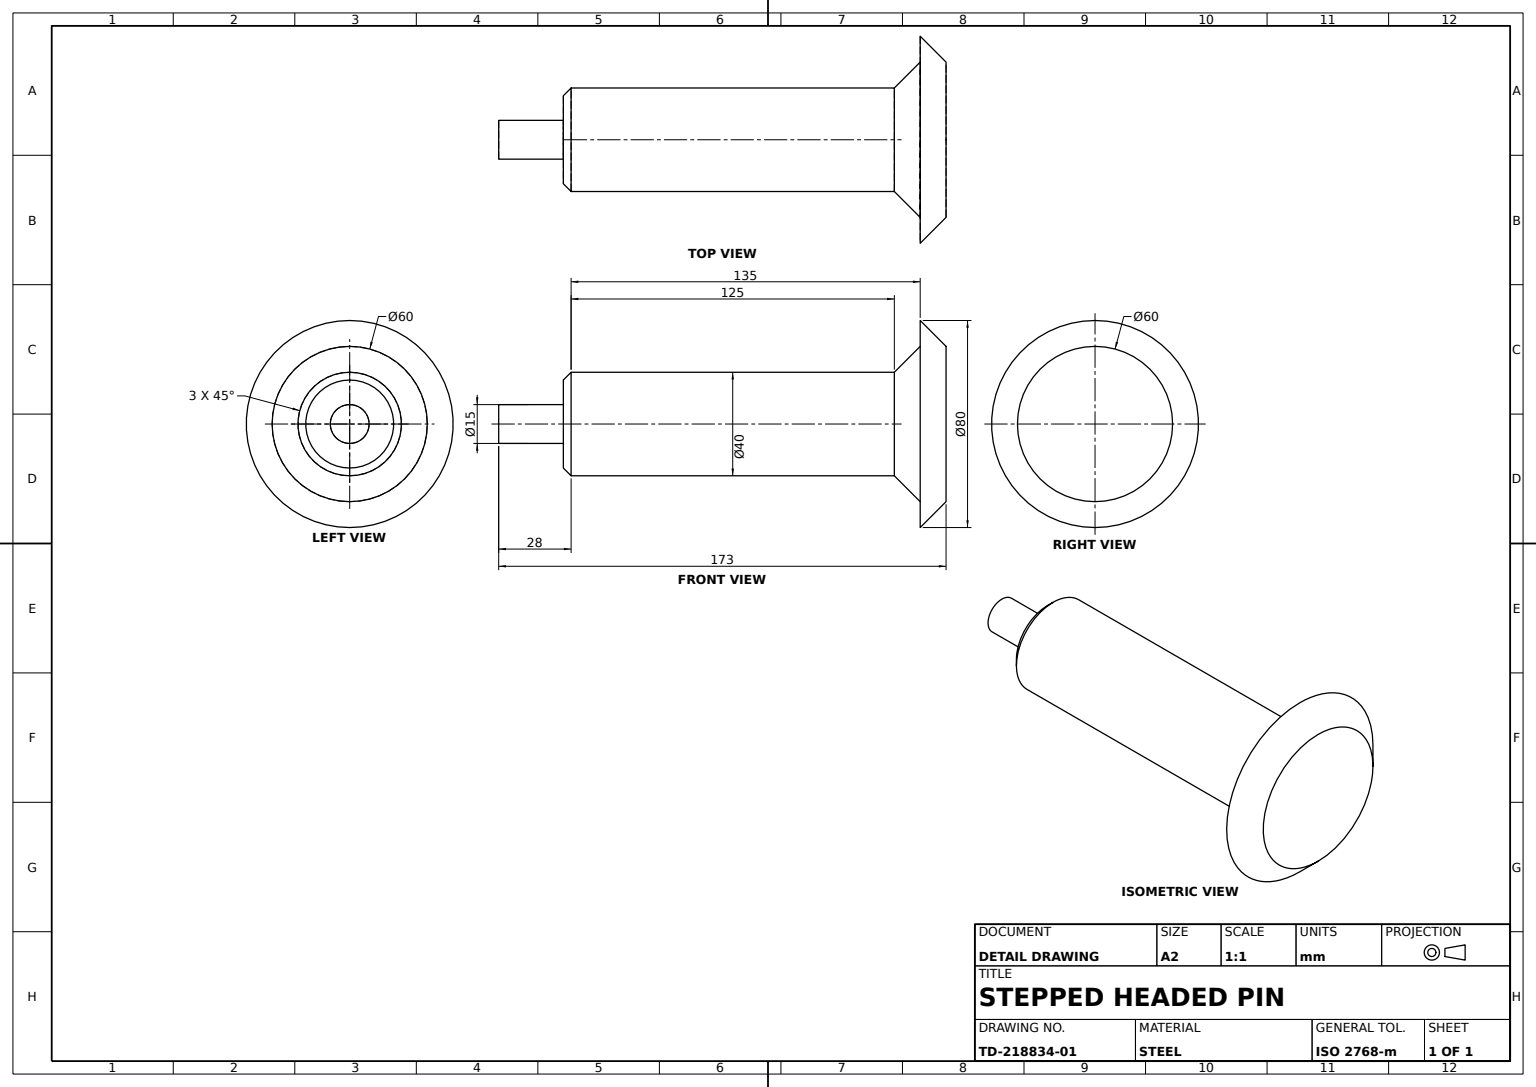
SolidWorks part; units mm, degrees
material "Plain Carbon Steel"
ref_plane "Front Plane" through (0, 0, 0) normal (0, 0, 1) x (1, 0, 0)
ref_plane "Top Plane" through (0, 0, 0) normal (0, 1, 0) x (1, 0, 0)
ref_plane "Right Plane" through (0, 0, 0) normal (1, 0, 0) x (0, 0, -1)
sketch "Pin Profile Sketch" plane through (0, 0, 0) normal (0, 0, 1) x (1, 0, 0)
  line L0 (213.2589, 0) -> (-138.2813, 0) construction
  line L1 (0, 20) -> (0, 0)
  line L3 (0, 20) -> (125, 20)
  line L4 (125, 20) -> (125, 0)
  line L5 (125, 20) -> (135, 30)
  line L6 (135, 0) -> (135, 40)
  line L7 (135, 40) -> (145, 30)
  line L8 (145, 30) -> (145, 0)
  line L10 (-3, 0) -> (-3, 17)
  line L11 (0, 20) -> (-3, 17)
  line L12 (-3, 7.5) -> (-28, 7.5)
  line L13 (-28, 7.5) -> (-28, 0)
  dimension "D1" = 125
  dimension "D2" = 135
  dimension "D3" = 145
  dimension "D4" = 3
  dimension "D5" = 28
  dimension "D6" = 40
  dimension "D7" = 7.5
  dimension "D8" = 9.5
  dimension "D9" = 3
  dimension "D10" = 10
  dimension "D11" = 45
  dimension "D12" = 20
  dimension "D13" = 30
  dimension "D14" = 40
  dimension "D15" = 7.5
revolve "Pin Body Revolve" add sketch "Pin Profile Sketch" angle 360 about L0
